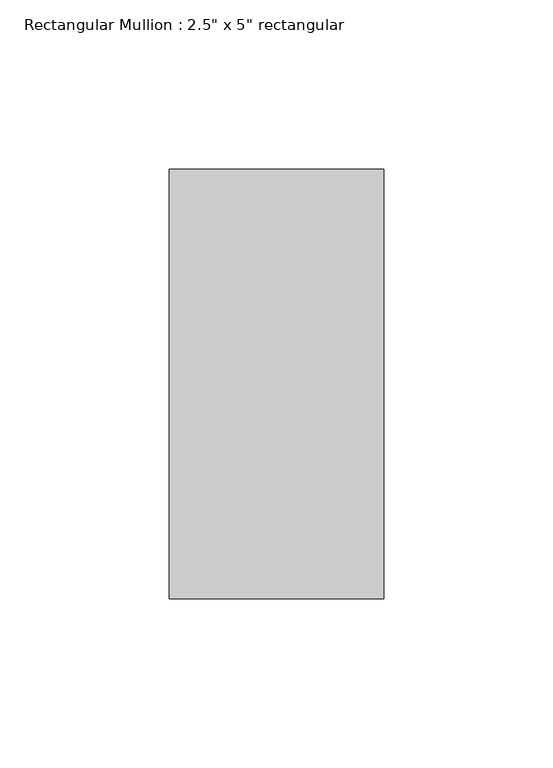
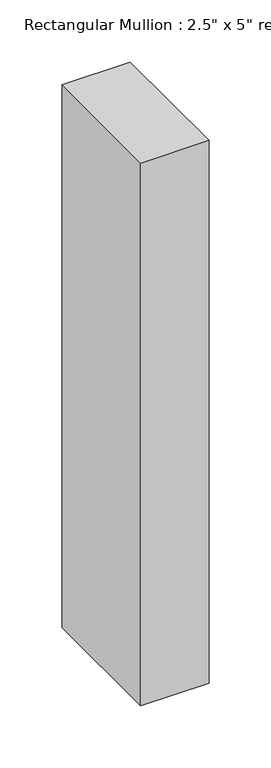
"""IFC4 building model written with IfcOpenShell, lengths in millimetres: member geometry."""

from ifc_helpers import new_model, si_unit, frame, origin, place, context, project, spatial, polyline, outline, extrude, source, transform, mapped, element, save


def member_bdfbb35d(model_context):
    return source(origin(), model_context, "Body", "SweptSolid", [
        extrude(outline(polyline([(31.75, 63.5), (31.75, -63.5), (-31.75, -63.5), (-31.75, 63.5), (31.75, 63.5)])), frame((0.0, 0.0, -533.4), z_axis=(0.0, 0.0, 1.0), x_axis=(1.0, 0.0, 0.0)), (0.0, 0.0, 1.0), 533.4),
    ])


if __name__ == "__main__":
    model = new_model("IFC4")
    model_context = context("Model", 3, world=origin())
    ifc_project = project(units=[si_unit("LENGTHUNIT", "METRE", prefix="MILLI")], contexts=[model_context])
    site = spatial("IfcSite", under=ifc_project)
    building = spatial("IfcBuilding", under=site)
    placement = place(None, origin())
    member_shape = member_bdfbb35d(model_context)
    element("IfcMember", 1, ObjectType="Rectangular Mullion : 2.5\" x 5\" rectangular", at=placement, inside=building, context=model_context, shape_type="MappedRepresentation", body=[
        mapped(member_shape, transform((0.0, 0.0, 0.0), x_axis=(1.0, 0.0, 0.0), y_axis=(0.0, 1.0, 0.0), z_axis=(0.0, 0.0, 1.0))),
    ])
    save(model, "model.ifc")

# Revit data of these elements
# Type "Rectangular Mullion : 2.5\" x 5\" rectangular"
#   built-in parameter 1007304 = 0.416667 (stored number, unit not read)
#   built-in parameter 1007301 = 0.104167 (stored number, unit not read)
#   built-in parameter 1007300 = 0.104167 (stored number, unit not read)
# Element 1 (IfcMember, "Rectangular Mullion : 2.5\" x 5\" rectangular")
#   Materials on its faces: "door colour"
# Materials
#   "door colour": class "Generic", colour RGB 120 120 120, transparency 0, Cost = 0
